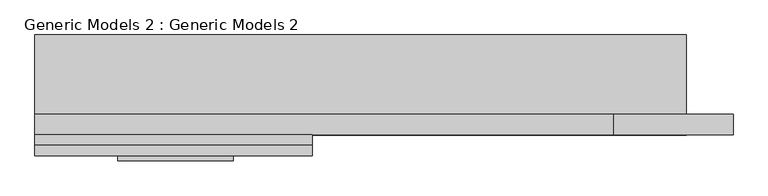
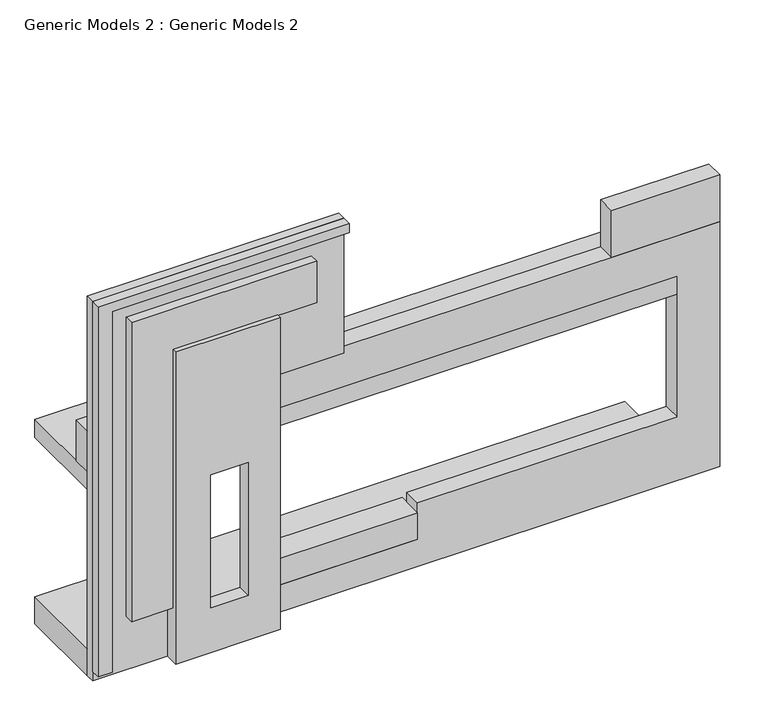
"""IFC4 building model written with IfcOpenShell, lengths in millimetres: proxy geometry, Generic Models 2 : Generic Models 2."""

from ifc_helpers import new_model, si_unit, frame, origin, place, context, project, spatial, polyline, outline, extrude, faceted_brep, source, transform, mapped, element, save


def generic_models_2_generic_models_2_88d393e9(model_context):
    return source(origin(), model_context, "Body", "SolidModel", [
        extrude(outline(polyline([(-8344.0529709, -15913.4200166), (-8344.0529709, -16218.2200166), (-10102.6718674, -16218.2200166), (-10102.6718674, -15913.4200166), (-8344.0529709, -15913.4200166)])), frame((0.0, 0.0, 7100.6641951), z_axis=(0.0, 0.0, 1.0), x_axis=(1.0, 0.0, 0.0)), (0.0, 0.0, 1.0), 808.6546252),
        extrude(outline(polyline([(-13260.9094994, -16218.2200166), (-15742.353759, -16218.2200166), (-15742.353759, -15786.4200166), (-13260.9094994, -15786.4200166), (-13260.9094994, -16218.2200166)])), frame((0.0, 0.0, 3352.8), z_axis=(0.0, 0.0, 1.0), x_axis=(1.0, 0.0, 0.0)), (0.0, 0.0, 1.0), 458.5624223),
        extrude(outline(polyline([(3048.0, -18633.0094994), (3048.0, -18404.4094994), (9263.5897688, -18404.4094994), (9263.5897688, -14543.4248841), (9420.6839376, -14543.4248841), (9420.6839376, -18633.0094994), (3048.0, -18633.0094994)])), frame((0.0, -16523.0200166, 0.0), z_axis=(0.0, 1.0, 0.0), x_axis=(0.0, 0.0, 1.0)), (0.0, 0.0, 1.0), 152.4),
        extrude(outline(polyline([(8960.2176833, -18086.9094994), (3811.3624223, -18086.9094994), (3811.3624223, -17413.1785039), (8249.0176833, -17413.1785039), (8249.0176833, -15076.3785039), (8960.2176833, -15076.3785039), (8960.2176833, -18086.9094994)])), frame((0.0, -16523.0200166, 0.0), z_axis=(0.0, 1.0, 0.0), x_axis=(0.0, 0.0, 1.0)), (0.0, 0.0, 1.0), 152.4),
        extrude(outline(polyline([(2888.2586619, -17413.1785039), (2888.2586619, -15710.5402465), (8261.3599231, -15710.5402465), (8261.3599231, -17413.1785039), (2888.2586619, -17413.1785039)]), holes=[polyline([(3658.9492475, -16232.7094994), (3658.9492475, -16842.3094994), (5944.9492475, -16842.3094994), (5944.9492475, -16232.7094994), (3658.9492475, -16232.7094994)])]), frame((0.0, -16599.2200166, 0.0), z_axis=(0.0, 1.0, 0.0), x_axis=(0.0, 0.0, 1.0)), (0.0, 0.0, 1.0), 228.6),
        extrude(outline(polyline([(9420.6839376, -18633.0094994), (2888.2586619, -18633.0094994), (2888.2586619, -17405.5991751), (7100.6641951, -17405.5991751), (7100.6641951, -14543.4248841), (9420.6839376, -14543.4248841), (9420.6839376, -18633.0094994)])), frame((0.0, -16370.6200166, 0.0), z_axis=(0.0, 1.0, 0.0), x_axis=(0.0, 0.0, 1.0)), (0.0, 0.0, 1.0), 152.4),
        faceted_brep([(-8344.0529709, -15911.7016107, 7100.6641951), (-8344.0529709, -16218.2200166, 7100.6641951), (-8344.0529709, -16218.2200166, 2888.2586619), (-8344.0529709, -15911.7016107, 2888.2586619), (-9031.8094994, -15913.4200166, 7100.6641951), (-9031.8094994, -15911.7016107, 7100.6641951), (-9031.8094994, -15911.7016107, 3352.8), (-9031.8094994, -15913.4200166, 3352.8), (-9031.8094994, -15913.4200166, 3978.3517748), (-9031.8094994, -16218.2200166, 3978.3517748), (-9031.8094994, -16218.2200166, 6400.8), (-9031.8094994, -15913.4200166, 6400.8), (-18633.0094994, -15913.4200166, 7100.6641951), (-18633.0094994, -16218.2200166, 7100.6641951), (-18633.0094994, -16218.2200166, 6400.8), (-13260.9094994, -16218.2200166, 3978.3517748), (-13260.9094994, -16218.2200166, 3352.8), (-18633.0094994, -16218.2200166, 3352.8), (-18633.0094994, -16218.2200166, 2888.2586619), (-18633.0094994, -14743.6805842, 2888.2586619), (-9031.8094994, -14743.6805842, 2888.2586619), (-9031.8094994, -15911.7016107, 2888.2586619), (-18633.0094994, -15913.4200166, 6400.8), (-9031.8094994, -14743.6805842, 3352.8), (-18633.0094994, -14743.6805842, 3352.8), (-13260.9094994, -15913.4200166, 3352.8), (-13260.9094994, -15913.4200166, 3978.3517748)], [[[0, 1, 2, 3]], [[4, 5, 6, 7, 8, 9, 10, 11]], [[1, 0, 5, 4, 12, 13]], [[2, 1, 13, 14, 10, 9, 15, 16, 17, 18]], [[3, 2, 18, 19, 20, 21]], [[0, 3, 21, 6, 5]], [[14, 22, 11, 10]], [[12, 4, 11, 22]], [[13, 12, 22, 14]], [[23, 20, 19, 24]], [[23, 24, 17, 16, 25, 7, 6]], [[18, 17, 24, 19]], [[20, 23, 6, 21]], [[15, 9, 8, 26]], [[26, 8, 7, 25]], [[15, 26, 25, 16]]]),
        extrude(outline(polyline([(-9031.8094994, -16218.2200166), (-18633.0094994, -16218.2200166), (-18633.0094994, -14743.6805842), (-9031.8094994, -14743.6805842), (-9031.8094994, -16218.2200166)])), frame((0.0, 0.0, 6096.0), z_axis=(0.0, 0.0, 1.0), x_axis=(1.0, 0.0, 0.0)), (0.0, 0.0, 1.0), 304.8),
    ])


if __name__ == "__main__":
    model = new_model("IFC4")
    model_context = context("Model", 3, world=origin())
    ifc_project = project(units=[si_unit("LENGTHUNIT", "METRE", prefix="MILLI")], contexts=[model_context])
    site = spatial("IfcSite", under=ifc_project)
    building = spatial("IfcBuilding", under=site)
    placement = place(None, origin())
    generic_models_2_generic_models_2_shape = generic_models_2_generic_models_2_88d393e9(model_context)
    element("IfcBuildingElementProxy", 1, Name="Generic Models 2 : Generic Models 2", ObjectType="Generic Models 2 : Generic Models 2", at=placement, inside=building, context=model_context, shape_type="MappedRepresentation", body=[
        mapped(generic_models_2_generic_models_2_shape, transform((0.0, 0.0, 0.0), x_axis=(1.0, 0.0, 0.0), y_axis=(0.0, 1.0, 0.0), z_axis=(0.0, 0.0, 1.0))),
    ])
    save(model, "model.ifc")
